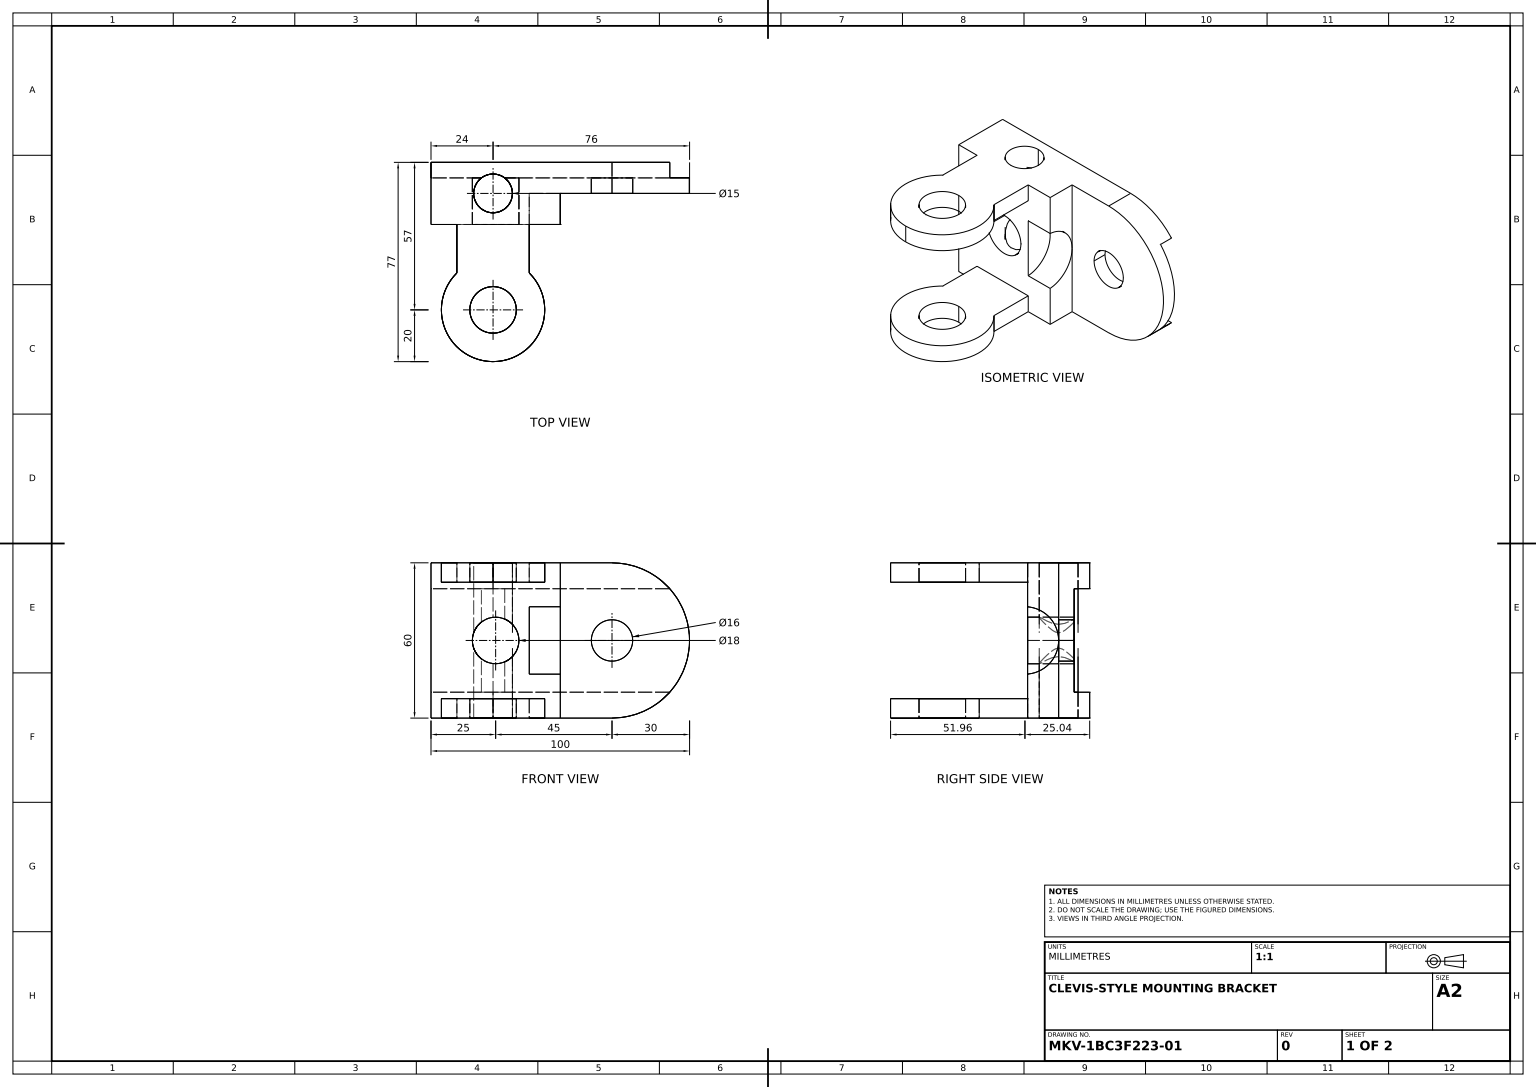
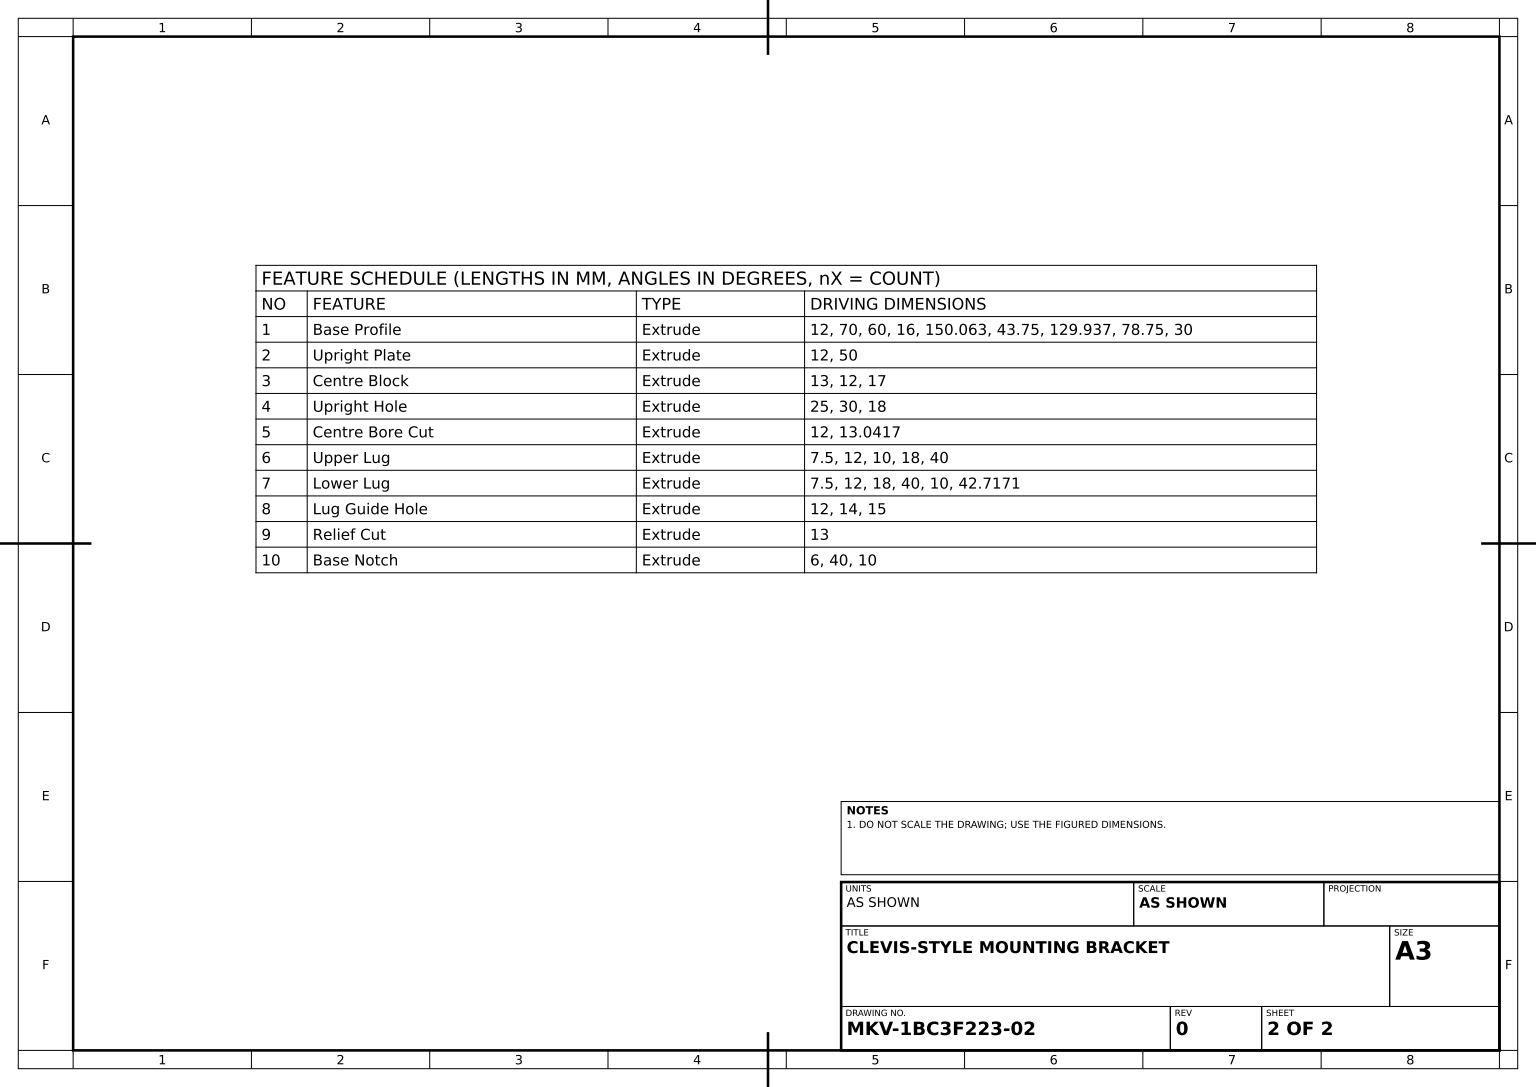
SolidWorks part; units mm, degrees
material "Plain Carbon Steel"
ref_plane "Front Plane" through (0, 0, 0) normal (0, 0, 1) x (1, 0, 0)
ref_plane "Top Plane" through (0, 0, 0) normal (0, 1, 0) x (1, 0, 0)
ref_plane "Right Plane" through (0, 0, 0) normal (1, 0, 0) x (0, 0, -1)
sketch "Base Profile Sketch" plane through (0, 0, 0) normal (0, 0, 1) x (1, 0, 0)
  line L0 (0, 0) -> (70, 0)
  line L1 (0, 0) -> (0, 60)
  line L2 (0, 60) -> (70, 60)
  line L4 (-43.75, 0) -> (106.3125, 0) construction
  line L5 (0, 78.75) -> (0, -51.1875) construction
  arc A0 (70, 60) -> (70, 0) centre (70, 30) cw
  circle A1 centre (70, 30) radius 8
  dimension "D3" = 70
  dimension "D4" = 16
  dimension "D1" = 70
  dimension "D2" = 60
  dimension "D5" = 30
  dimension "D6" = 150.0625
  dimension "D7" = 43.75
  dimension "D8" = 129.9375
  dimension "D9" = 78.75
  dimension "D10" = 30
extrude "Base Profile" add sketch "Base Profile Sketch" along normal mid plane 12
sketch "Upright Plate Sketch" plane through (0, 0, 6) normal (0, 0, 1) x (1, 0, 0)
  line L0 (0, 60) -> (0, 0)
  line L1 (0, 0) -> (50, 0)
  line L2 (0, 0) -> (70, 0) construction
  line L3 (50, 0) -> (50, 60)
  line L4 (70, 60) -> (0, 60) construction
  line L5 (50, 60) -> (0, 60)
  dimension "D1" = 50
extrude "Upright Plate" add sketch "Upright Plate Sketch" along normal blind 12
sketch "Centre Block Sketch" plane through (0, 0, 18) normal (0, 0, 1) x (1, 0, 0)
  line L0 (50, 0) -> (50, 17)
  line L1 (50, 0) -> (50, 60) construction
  line L2 (50, 17) -> (38, 17)
  line L3 (38, 17) -> (38, 0)
  line L4 (0, 0) -> (50, 0) construction
  line L5 (38, 0) -> (50, 0)
  line L6 (50, 60) -> (38, 60)
  line L7 (50, 60) -> (0, 60) construction
  line L8 (38, 60) -> (38, 43)
  line L9 (38, 43) -> (50, 43)
  line L10 (50, 0) -> (50, 60) construction
  line L11 (50, 43) -> (50, 60)
  dimension "D1" = 12
  dimension "D2" = 12
  dimension "D3" = 17
  dimension "D4" = 17
extrude "Centre Block" add sketch "Centre Block Sketch" along normal blind 13
sketch "Upright Hole Sketch" plane through (0, 0, 18) normal (0, 0, 1) x (1, 0, 0)
  line L0 (0, 60) -> (0, 0) construction
  circle A0 centre (25, 30) radius 9
  dimension "D3" = 18
  dimension "D1" = 25
  dimension "D2" = 30
extrude "Upright Hole" cut sketch "Upright Hole Sketch" against normal through all
sketch "Centre Bore Sketch" plane through (50, 0, 0) normal (1, 0, 0) x (0, 0, -1)
  arc A0 (-18, 43) -> (-18, 17) centre (-19.0417, 30) cw
  dimension "D1" = 13.0417
extrude "Centre Bore Cut" cut sketch "Centre Bore Sketch" against normal blind 12 and the other way through all flip side to cut
sketch "Upper Lug Sketch" plane through (0, 0, 0) normal (0, -1, 0) x (1, 0, 0)
  line L0 (0, -6) -> (0, 6)
  line L1 (0, 18) -> (0, -6) construction
  line L2 (0, 6) -> (10, 6)
  line L3 (10, 6) -> (10, 36.7171)
  line L4 (38, 36.7171) -> (38, -6)
  line L5 (38, 36.7171) -> (38, 31)
  line L6 (38, 31) -> (50, 31) construction
  line L7 (0, -6) -> (70, -6) construction
  line L8 (38, -6) -> (0, -6)
  arc A0 (38, 36.7171) -> (10, 36.7171) centre (24, 51) ccw
  circle A1 centre (24, 51) radius 9
  line M5 (0, -6) -> (70, -6)
  line M10 (38, 31) -> (38, 18)
  line M11 (38, 18) -> (0, 18)
  line M12 (0, 18) -> (0, -6)
  dimension "D5" = 18
  dimension "D6" = 40
  dimension "D1" = 12
  dimension "D2" = 10
  dimension "D4" = 14
extrude "Upper Lug" add sketch "Upper Lug Sketch" against normal blind 7.5 contours L4 L3 L2 M11 M12 M5 | L4 A0 L3 A1 M11 M10
sketch "Lower Lug Sketch" plane through (0, 60, 0) normal (0, 1, 0) x (1, 0, 0)
  line L0 (0, 6) -> (0, -6)
  line L1 (0, -18) -> (0, 6) construction
  line L2 (0, -6) -> (10, -6)
  line L7 (38, -36.7171) -> (38, 6)
  line L8 (70, 6) -> (0, 6) construction
  line L9 (38, 6) -> (0, 6)
  line L10 (10, -6) -> (10, -36.7171)
  circle A0 centre (24, -51) radius 9
  arc A1 (10, -36.7171) -> (38, -36.7171) centre (24, -51) ccw
  dimension "D4" = 18
  dimension "D6" = 40
  dimension "D1" = 12
  dimension "D2" = 10
  dimension "D3" = 42.7171
  dimension "D5" = 70
extrude "Lower Lug" add sketch "Lower Lug Sketch" against normal blind 7.5
sketch "Lug Guide Hole Sketch" plane through (0, 0, 0) normal (0, -1, 0) x (1, 0, 0)
  line L0 (0, -6) -> (70, -6) construction
  line L2 (10, 18) -> (10, 36.7171) construction
  circle A0 centre (24, 6) radius 7.5
  dimension "D3" = 15
  dimension "D1" = 12
  dimension "D2" = 14
extrude "Lug Guide Hole" cut sketch "Lug Guide Hole Sketch" against normal through all
sketch "Relief Cut Sketch" plane through (0, 0, 31) normal (0, 0, 1) x (1, 0, 0)
  line L0 (38, 43) -> (50, 43)
  line L1 (50, 43) -> (50, 60)
  line L2 (50, 60) -> (38, 60)
  line L3 (38, 60) -> (38, 43)
  line L4 (38, 17) -> (50, 17)
  line L5 (50, 17) -> (50, 0)
  line L6 (38, 17) -> (38, 0)
  line L7 (38, 0) -> (50, 0)
extrude "Relief Cut" cut sketch "Relief Cut Sketch" against normal blind 13 contours L3 L0 L1 L2 | L7 L5 L4 L6
sketch "Base Notch Sketch" plane through (0, 0, 0) normal (-1, 0, 0) x (0, 0, 1)
  line L0 (-6, 50) -> (0, 50)
  line L1 (-6, 60) -> (-6, 0) construction
  line L2 (0, 50) -> (0, 10)
  line L3 (0, 10) -> (-6, 10)
  line L4 (-6, 10) -> (-6, 50)
  dimension "D1" = 6
  dimension "D2" = 40
  dimension "D3" = 10
extrude "Base Notch" cut sketch "Base Notch Sketch" against normal through all
